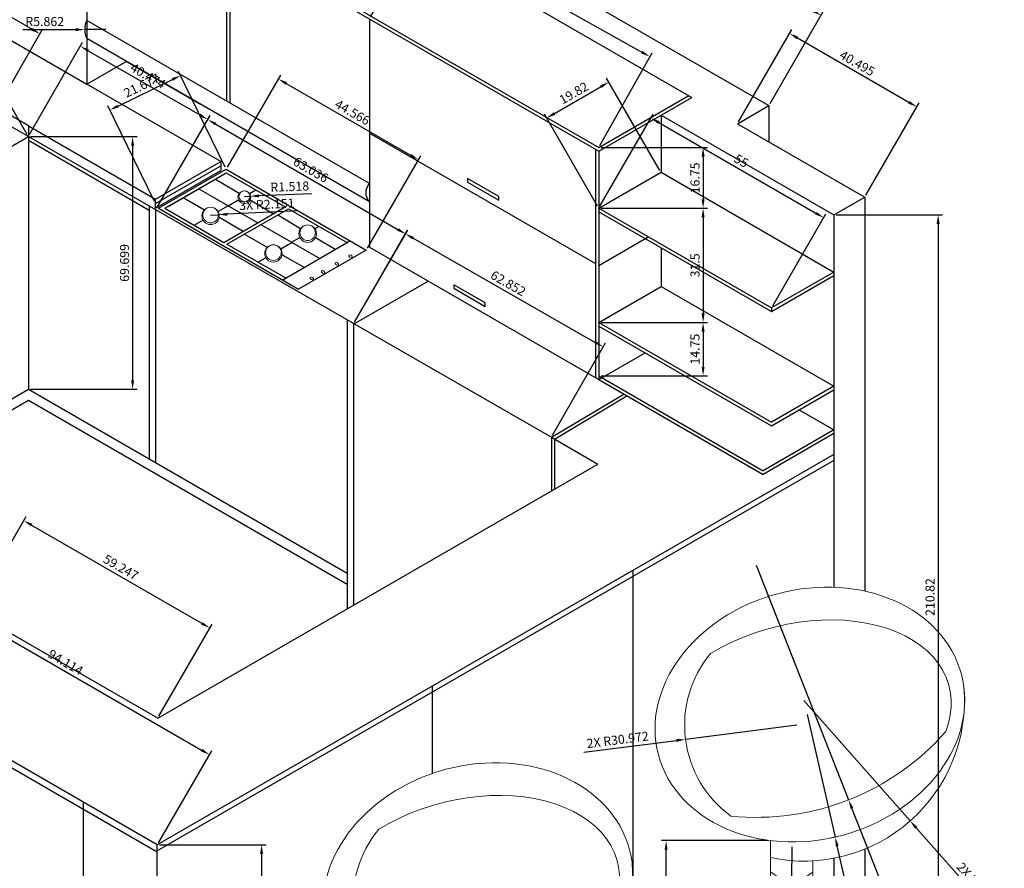
# Model space of a CAD drawing. Units: centimetres. Extents: x 239489 to 240034, y 95136 to 95693.
# Tile 3 of 4: x 239762 to 240034, y 95322 to 95556. Entities that reach past the tile are written whole.
import ezdxf

# ---------------------------------------------------------------- set-up
doc = ezdxf.new("R2010")
doc.units = ezdxf.units.CM
for name, color, linetype, lineweight in [('A-ANNO-DIMS', 2, 'Continuous', 18), ('A-EQPM', 8, 'Continuous', 18), ('A-FLOR-CASE', 7, 'Continuous', 25), ('A-FURN', 8, 'Continuous', 18)]:
    doc.layers.add(name, color=color, linetype=linetype, lineweight=lineweight)
doc.styles.get("Standard").update_dxf_attribs({"font": 'arial.ttf'})
doc.dimstyles.new('ISO-25', dxfattribs={"dimtxt": 2.5, "dimasz": 2.5, "dimexe": 1.25, "dimexo": 0.625, "dimtad": 1, "dimdec": 1, "dimdsep": 46, "dimtxsty": 'Standard', "dimcen": 2.5, "dimadec": 0, "dimazin": 0, "dimtfac": 1, "dimtdec": 1, "dimtmove": 0, "dimatfit": 3, "dimfxl": 1, "dimarcsym": 0})

# ---------------------------------------------------------------- blocks, each defined once
blk = doc.blocks.new('chair')
for p, q in [((240038.62, 95198.57), (240038.62, 95083.6)), ((240050.31, 95192.98), (240050.31, 95083.6))]:
    blk.add_line(p, q)
for centre, radius, start, end in [((240045.95, 95230.38), 30.97, 140.3765, 234.0123), ((240047.85, 95237.18), 44.27, 257.9755, 4.8871), ((240034.71, 95274.51), 69.54, 264.2585, 318.7167), ((240048.77, 95233.37), 34.72, 279.5939, 286.053), ((240044.52, 95196.85), 9.07, 229.4992, 309.6922), ((240044.46, 95080.37), 6.67, 151.0567, 28.8701), ((240044.47, 95082.04), 6.05, 165.0328, 14.894), ((240044.47, 95086.14), 6.37, 203.4476, 336.4791)]:
    blk.add_arc(centre, radius, start, end)
blk.add_ellipse((240049.51, 95233.34), major_axis=(41.76, 11.11), ratio=0.798178)
for centre, major_axis, ratio, start_param, end_param in [((240046.12, 95230.16), (41.76, 11.11), 0.649156, 5.842129, 8.285652), ((240044.64, 95075.07), (-24.53, 0), 0.903861, 4.9602, 10.762393)]:
    blk.add_ellipse(centre, major_axis=major_axis, ratio=ratio, start_param=start_param, end_param=end_param)
for points, knots in [([(240050.31, 95149.47), (240053.45, 95154.4), (240062.71, 95168.9), (240023.27, 95171.77), (240016.58, 95146.62), (240022.37, 95124.99), (240049.4, 95122.25), (240052.18, 95137.64), (240053.6, 95145.49)], [0, 0, 0, 0, 14.382035, 42.295085, 64.991841, 82.938136, 102.944135, 123.773993, 123.773993, 123.773993, 123.773993]), ([(240050.31, 95151.33), (240050.86, 95152.21), (240051.4, 95153.07), (240052.67, 95155.21), (240053.34, 95156.46), (240054.37, 95158.8), (240054.7, 95159.88), (240054.88, 95161.29), (240054.88, 95161.73), (240054.77, 95162.52), (240054.66, 95162.88), (240054.32, 95163.58), (240054.09, 95163.91), (240053.51, 95164.56), (240053.15, 95164.87), (240051.85, 95165.79), (240050.7, 95166.33), (240048.02, 95167.17), (240046.5, 95167.47), (240043.26, 95167.81), (240041.54, 95167.85), (240037.24, 95167.61), (240034.64, 95167.17), (240031.24, 95166.1), (240030.23, 95165.71), (240027.8, 95164.52), (240026.51, 95163.63), (240024.3, 95161.56), (240023.38, 95160.4), (240021.86, 95157.85), (240021.25, 95156.46), (240019.83, 95151.95), (240019.48, 95148.58), (240019.62, 95142.56), (240019.95, 95139.94), (240021.18, 95135.59), (240021.97, 95133.78), (240023.74, 95131.18), (240024.56, 95130.25), (240026.17, 95128.89), (240026.88, 95128.4), (240028.41, 95127.53), (240029.24, 95127.14), (240032.19, 95126.03), (240034.5, 95125.58), (240038.99, 95125.46), (240041.16, 95125.78), (240043.66, 95126.75), (240044.27, 95127.05), (240045.4, 95127.76), (240045.91, 95128.16), (240047.34, 95129.53), (240048.14, 95130.64), (240049.5, 95133.2), (240050.06, 95134.65), (240050.79, 95137.03), (240051.02, 95137.89), (240051.24, 95138.77)], [1.291453, 1.291453, 1.291453, 1.291453, 3.859328, 3.859328, 7.768299, 7.768299, 11.677271, 11.677271, 13.651412, 13.651412, 15.625553, 15.625553, 17.599694, 17.599694, 19.573836, 19.573836, 23.79302, 23.79302, 28.012204, 28.012204, 32.231389, 32.231389, 38.538282, 38.538282, 41.377864, 41.377864, 45.999792, 45.999792, 50.62172, 50.62172, 55.243647, 55.243647, 64.836636, 64.836636, 72.329787, 72.329787, 78.440683, 78.440683, 82.448991, 82.448991, 85.126657, 85.126657, 87.804323, 87.804323, 94.31242, 94.31242, 100.820517, 100.820517, 103.180094, 103.180094, 105.53967, 105.53967, 110.270519, 110.270519, 115.001369, 115.001369, 117.513572, 117.513572, 117.513572, 117.513572]), ([(240038.62, 95150.05), (240037.1, 95148.99), (240030.34, 95144.28), (240045.99, 95138.79), (240055.45, 95146.41), (240051.11, 95148.83), (240050.31, 95149.47)], [0, 0, 0, 0, 4.688566, 20.875909, 24.405284, 27.513147, 27.513147, 27.513147, 27.513147]), ([(240038.62, 95145.45), (240038.41, 95145.3), (240038.2, 95145.16), (240037.99, 95145.01), (240036.47, 95143.95), (240029.7, 95139.25), (240045.36, 95133.75), (240054.55, 95141.16), (240051.25, 95143.33), (240050.31, 95143.98)], [-0.650979, -0.650979, -0.650979, -0.650979, 0, 0, 0, 4.688566, 20.875909, 24.405284, 26.869866, 26.869866, 26.869866, 26.869866])]:
    blk.add_open_spline(points, degree=3, knots=knots)
blk = doc.blocks.new('HANDLE-DOOR')
for p, q in [((0.87, 10.5), (0, 10)), ((0, 10), (0, 0)), ((0.87, 0.5), (0.87, 10.5)), ((0, 0), (0.87, 0.5))]:
    blk.add_line(p, q)
blk = doc.blocks.new('*D5')
at = {"layer": 'A-ANNO-DIMS', "color": 0, "lineweight": -2, "transparency": 16777216}
for p, q in [((239735.57, 95667.89), (239750.25, 95693.33)), ((239751.79, 95691), (239980.86, 95558.75)), ((239968.97, 95533.14), (239983.65, 95558.58))]:
    blk.add_line(p, q, dxfattribs=at)
at = {"layer": 'A-ANNO-DIMS', "color": 0, "transparency": 16777216}
for points in [[(239752, 95691.36), (239751.59, 95690.64), (239749.63, 95692.25)], [(239981.07, 95559.11), (239980.65, 95558.39), (239983.03, 95557.5)]]:
    blk.add_solid(points, dxfattribs=at)
at = {"layer": 'Defpoints', "color": 0, "transparency": 16777216}
for p in [(239735.25, 95667.35), (239983.03, 95557.5), (239968.65, 95532.6)]:
    blk.add_point(p, dxfattribs=at)
at = {"layer": 'A-ANNO-DIMS', "color": 0, "transparency": 16777216, "insert": (239867.28, 95626.52), "char_height": 2.5, "attachment_point": 5, "rotation": 330}
blk.add_mtext('269.505', dxfattribs=at)
blk = doc.blocks.new('*D6')
at = {"layer": 'A-ANNO-DIMS', "color": 0, "lineweight": -2, "transparency": 16777216}
for p, q in [((239960.31, 95528.14), (239974.99, 95553.58)), ((239976.53, 95551.25), (240007.27, 95533.5)), ((239995.37, 95507.89), (240010.06, 95533.33))]:
    blk.add_line(p, q, dxfattribs=at)
at = {"layer": 'A-ANNO-DIMS', "color": 0, "transparency": 16777216}
for points in [[(239976.74, 95551.61), (239976.32, 95550.89), (239974.37, 95552.5)], [(240007.48, 95533.86), (240007.06, 95533.14), (240009.44, 95532.25)]]:
    blk.add_solid(points, dxfattribs=at)
at = {"layer": 'Defpoints', "color": 0, "transparency": 16777216}
for p in [(240009.44, 95532.25), (239959.99, 95527.6), (239995.06, 95507.35)]:
    blk.add_point(p, dxfattribs=at)
at = {"layer": 'A-ANNO-DIMS', "color": 0, "transparency": 16777216, "insert": (239992.85, 95544.02), "char_height": 2.5, "attachment_point": 5, "rotation": 330}
blk.add_mtext('40.495', dxfattribs=at)
blk = doc.blocks.new('*D9')
at = {"layer": 'A-ANNO-DIMS', "color": 0, "lineweight": -2, "transparency": 16777216}
for p, q in [((239987.18, 95502.44), (240016.56, 95502.44)), ((240015.31, 95499.94), (240015.31, 95294.12)), ((239987.18, 95291.62), (240016.56, 95291.62))]:
    blk.add_line(p, q, dxfattribs=at)
at = {"layer": 'A-ANNO-DIMS', "color": 0, "transparency": 16777216}
for points in [[(240014.89, 95499.94), (240015.73, 95499.94), (240015.31, 95502.44)], [(240014.89, 95294.12), (240015.73, 95294.12), (240015.31, 95291.62)]]:
    blk.add_solid(points, dxfattribs=at)
at = {"layer": 'Defpoints', "color": 0, "transparency": 16777216}
for p in [(239986.56, 95502.44), (239986.56, 95291.62), (240015.31, 95291.62)]:
    blk.add_point(p, dxfattribs=at)
at = {"layer": 'A-ANNO-DIMS', "color": 0, "transparency": 16777216, "insert": (240013.41, 95397.03), "char_height": 2.5, "attachment_point": 5, "rotation": 90}
blk.add_mtext('210.82', dxfattribs=at)
blk = doc.blocks.new('*D24')
at = {"layer": 'A-ANNO-DIMS', "color": 0, "lineweight": -2, "transparency": 16777216}
for p, q in [((239858.85, 95557.08), (239873.23, 95582.69)), ((239874.8, 95580.37), (239933.66, 95547.32)), ((239922.07, 95521.58), (239936.45, 95547.19))]:
    blk.add_line(p, q, dxfattribs=at)
at = {"layer": 'A-ANNO-DIMS', "color": 0, "transparency": 16777216}
for points in [[(239875, 95580.74), (239874.6, 95580.01), (239872.62, 95581.6)], [(239933.86, 95547.69), (239933.46, 95546.96), (239935.84, 95546.1)]]:
    blk.add_solid(points, dxfattribs=at)
at = {"layer": 'Defpoints', "color": 0, "transparency": 16777216}
for p in [(239858.54, 95556.53), (239935.84, 95546.1), (239921.76, 95521.03)]:
    blk.add_point(p, dxfattribs=at)
at = {"layer": 'A-ANNO-DIMS', "color": 0, "transparency": 16777216, "insert": (239905.16, 95565.51), "char_height": 2.5, "attachment_point": 5, "rotation": 330.6844}
blk.add_mtext('72.505', dxfattribs=at)
blk = doc.blocks.new('*D25')
at = {"layer": 'A-ANNO-DIMS', "color": 0, "lineweight": -2, "transparency": 16777216}
for p, q in [((239922.39, 95521.03), (239951.76, 95521.03)), ((239950.51, 95518.53), (239950.51, 95506.78)), ((239922.39, 95504.28), (239951.76, 95504.28))]:
    blk.add_line(p, q, dxfattribs=at)
at = {"layer": 'A-ANNO-DIMS', "color": 0, "transparency": 16777216}
for points in [[(239950.1, 95518.53), (239950.93, 95518.53), (239950.51, 95521.03)], [(239950.1, 95506.78), (239950.93, 95506.78), (239950.51, 95504.28)]]:
    blk.add_solid(points, dxfattribs=at)
at = {"layer": 'Defpoints', "color": 0, "transparency": 16777216}
for p in [(239921.76, 95521.03), (239921.76, 95504.28), (239950.51, 95504.28)]:
    blk.add_point(p, dxfattribs=at)
at = {"layer": 'A-ANNO-DIMS', "color": 0, "transparency": 16777216, "insert": (239948.61, 95512.66), "char_height": 2.5, "attachment_point": 5, "rotation": 90}
blk.add_mtext('16.75', dxfattribs=at)
blk = doc.blocks.new('*D26')
at = {"layer": 'A-ANNO-DIMS', "color": 0, "lineweight": -2, "transparency": 16777216}
for p, q in [((239922.39, 95504.28), (239951.76, 95504.28)), ((239950.51, 95501.78), (239950.51, 95475.28)), ((239922.39, 95472.78), (239951.76, 95472.78))]:
    blk.add_line(p, q, dxfattribs=at)
at = {"layer": 'A-ANNO-DIMS', "color": 0, "transparency": 16777216}
for points in [[(239950.1, 95501.78), (239950.93, 95501.78), (239950.51, 95504.28)], [(239950.1, 95475.28), (239950.93, 95475.28), (239950.51, 95472.78)]]:
    blk.add_solid(points, dxfattribs=at)
at = {"layer": 'Defpoints', "color": 0, "transparency": 16777216}
for p in [(239921.76, 95504.28), (239921.76, 95472.78), (239950.51, 95472.78)]:
    blk.add_point(p, dxfattribs=at)
at = {"layer": 'A-ANNO-DIMS', "color": 0, "transparency": 16777216, "insert": (239948.61, 95488.53), "char_height": 2.5, "attachment_point": 5, "rotation": 90}
blk.add_mtext('31.5', dxfattribs=at)
blk = doc.blocks.new('*D27')
at = {"layer": 'A-ANNO-DIMS', "color": 0, "lineweight": -2, "transparency": 16777216}
for p, q in [((239922.39, 95472.78), (239951.76, 95472.78)), ((239950.51, 95470.28), (239950.51, 95460.53)), ((239922.39, 95458.03), (239951.76, 95458.03))]:
    blk.add_line(p, q, dxfattribs=at)
at = {"layer": 'A-ANNO-DIMS', "color": 0, "transparency": 16777216}
for points in [[(239950.1, 95470.28), (239950.93, 95470.28), (239950.51, 95472.78)], [(239950.1, 95460.53), (239950.93, 95460.53), (239950.51, 95458.03)]]:
    blk.add_solid(points, dxfattribs=at)
at = {"layer": 'Defpoints', "color": 0, "transparency": 16777216}
for p in [(239921.76, 95472.78), (239921.76, 95458.03), (239950.51, 95458.03)]:
    blk.add_point(p, dxfattribs=at)
at = {"layer": 'A-ANNO-DIMS', "color": 0, "transparency": 16777216, "insert": (239948.61, 95465.41), "char_height": 2.5, "attachment_point": 5, "rotation": 90}
blk.add_mtext('14.75', dxfattribs=at)
blk = doc.blocks.new('*D28')
at = {"layer": 'A-ANNO-DIMS', "color": 0, "lineweight": -2, "transparency": 16777216}
for p, q in [((239922.08, 95504.82), (239936.76, 95530.26)), ((239938.3, 95527.93), (239981.6, 95502.93)), ((239969.71, 95477.32), (239984.39, 95502.76))]:
    blk.add_line(p, q, dxfattribs=at)
at = {"layer": 'A-ANNO-DIMS', "color": 0, "transparency": 16777216}
for points in [[(239938.51, 95528.29), (239938.09, 95527.57), (239936.14, 95529.18)], [(239981.81, 95503.29), (239981.4, 95502.57), (239983.77, 95501.68)]]:
    blk.add_solid(points, dxfattribs=at)
at = {"layer": 'Defpoints', "color": 0, "transparency": 16777216}
for p in [(239921.76, 95504.28), (239983.77, 95501.68), (239969.39, 95476.78)]:
    blk.add_point(p, dxfattribs=at)
at = {"layer": 'A-ANNO-DIMS', "color": 0, "transparency": 16777216, "insert": (239960.9, 95517.07), "char_height": 2.5, "attachment_point": 5, "rotation": 330}
blk.add_mtext('55', dxfattribs=at)
blk = doc.blocks.new('*D29')
at = {"layer": 'A-ANNO-DIMS', "color": 0, "lineweight": -2, "transparency": 16777216}
for p, q in [((239938.61, 95514.73), (239923.93, 95540.17)), ((239909.55, 95530.43), (239922.39, 95537.84)), ((239921.45, 95504.82), (239906.76, 95530.26))]:
    blk.add_line(p, q, dxfattribs=at)
at = {"layer": 'A-ANNO-DIMS', "color": 0, "transparency": 16777216}
for points in [[(239922.18, 95538.2), (239922.6, 95537.48), (239924.55, 95539.09)], [(239909.34, 95530.79), (239909.76, 95530.07), (239907.39, 95529.18)]]:
    blk.add_solid(points, dxfattribs=at)
at = {"layer": 'Defpoints', "color": 0, "transparency": 16777216}
for p in [(239924.55, 95539.09), (239938.93, 95514.19), (239921.76, 95504.28)]:
    blk.add_point(p, dxfattribs=at)
at = {"layer": 'A-ANNO-DIMS', "color": 0, "transparency": 16777216, "insert": (239915.02, 95535.78), "char_height": 2.5, "attachment_point": 5, "rotation": 30}
blk.add_mtext('19.82', dxfattribs=at)
blk = doc.blocks.new('*D32')
at = {"layer": 'A-ANNO-DIMS', "color": 0, "lineweight": -2, "transparency": 16777216}
for p, q in [((239764.18, 95524.59), (239749.49, 95550.03)), ((239697.39, 95518.51), (239747.95, 95547.7)), ((239709.29, 95492.9), (239694.6, 95518.34))]:
    blk.add_line(p, q, dxfattribs=at)
at = {"layer": 'A-ANNO-DIMS', "color": 0, "transparency": 16777216}
for points in [[(239747.75, 95548.06), (239748.16, 95547.34), (239750.12, 95548.95)], [(239697.19, 95518.87), (239697.6, 95518.15), (239695.23, 95517.26)]]:
    blk.add_solid(points, dxfattribs=at)
at = {"layer": 'Defpoints', "color": 0, "transparency": 16777216}
for p in [(239750.12, 95548.95), (239764.49, 95524.05), (239709.6, 95492.36)]:
    blk.add_point(p, dxfattribs=at)
at = {"layer": 'A-ANNO-DIMS', "color": 0, "transparency": 16777216, "insert": (239721.72, 95534.75), "char_height": 2.5, "attachment_point": 5, "rotation": 30}
blk.add_mtext('63.381', dxfattribs=at)
blk = doc.blocks.new('*D33')
at = {"layer": 'A-ANNO-DIMS', "color": 0, "lineweight": -2, "transparency": 16777216}
for p, q in [((239764.81, 95524.59), (239779.45, 95550.06)), ((239781, 95547.73), (239811.75, 95530.04)), ((239799.89, 95504.41), (239814.54, 95529.87))]:
    blk.add_line(p, q, dxfattribs=at)
at = {"layer": 'A-ANNO-DIMS', "color": 0, "transparency": 16777216}
for points in [[(239781.21, 95548.09), (239780.79, 95547.36), (239778.83, 95548.97)], [(239811.95, 95530.4), (239811.54, 95529.67), (239813.91, 95528.79)]]:
    blk.add_solid(points, dxfattribs=at)
at = {"layer": 'Defpoints', "color": 0, "transparency": 16777216}
for p in [(239813.91, 95528.79), (239764.49, 95524.05), (239799.58, 95503.87)]:
    blk.add_point(p, dxfattribs=at)
at = {"layer": 'A-ANNO-DIMS', "color": 0, "transparency": 16777216, "insert": (239797.32, 95540.53), "char_height": 2.5, "attachment_point": 5, "rotation": 330.0888}
blk.add_mtext('40.474', dxfattribs=at)
blk = doc.blocks.new('*D34')
at = {"layer": 'A-ANNO-DIMS', "color": 0, "lineweight": -2, "transparency": 16777216}
for p, q in [((239799.89, 95504.41), (239814.6, 95529.83)), ((239816.14, 95527.5), (239866.37, 95498.43)), ((239854.45, 95472.84), (239869.16, 95498.26))]:
    blk.add_line(p, q, dxfattribs=at)
at = {"layer": 'A-ANNO-DIMS', "color": 0, "transparency": 16777216}
for points in [[(239816.35, 95527.86), (239815.93, 95527.14), (239813.98, 95528.75)], [(239866.58, 95498.79), (239866.16, 95498.07), (239868.54, 95497.18)]]:
    blk.add_solid(points, dxfattribs=at)
at = {"layer": 'Defpoints', "color": 0, "transparency": 16777216}
for p in [(239799.58, 95503.87), (239868.54, 95497.18), (239854.14, 95472.3)]:
    blk.add_point(p, dxfattribs=at)
at = {"layer": 'A-ANNO-DIMS', "color": 0, "transparency": 16777216, "insert": (239842.21, 95514.61), "char_height": 2.5, "attachment_point": 5, "rotation": 329.943}
blk.add_mtext('63.036', dxfattribs=at)
blk = doc.blocks.new('*D35')
at = {"layer": 'A-ANNO-DIMS', "color": 0, "lineweight": -2, "transparency": 16777216}
for p, q in [((239854.45, 95472.84), (239869.03, 95498.34)), ((239870.58, 95496.01), (239920.8, 95467.29)), ((239909.01, 95441.64), (239923.59, 95467.14))]:
    blk.add_line(p, q, dxfattribs=at)
at = {"layer": 'A-ANNO-DIMS', "color": 0, "transparency": 16777216}
for points in [[(239870.79, 95496.37), (239870.37, 95495.65), (239868.41, 95497.25)], [(239921.01, 95467.65), (239920.59, 95466.93), (239922.97, 95466.05)]]:
    blk.add_solid(points, dxfattribs=at)
at = {"layer": 'Defpoints', "color": 0, "transparency": 16777216}
for p in [(239854.14, 95472.3), (239922.97, 95466.05), (239908.7, 95441.09)]:
    blk.add_point(p, dxfattribs=at)
at = {"layer": 'A-ANNO-DIMS', "color": 0, "transparency": 16777216, "insert": (239896.63, 95483.3), "char_height": 2.5, "attachment_point": 5, "rotation": 330.235}
blk.add_mtext('62.852', dxfattribs=at)
blk = doc.blocks.new('*D36')
at = {"layer": 'A-ANNO-DIMS', "color": 0, "lineweight": -2, "transparency": 16777216}
for p, q in [((239765.12, 95524.05), (239794.49, 95524.05)), ((239793.24, 95521.55), (239793.24, 95456.85)), ((239765.12, 95454.35), (239794.49, 95454.35))]:
    blk.add_line(p, q, dxfattribs=at)
at = {"layer": 'A-ANNO-DIMS', "color": 0, "transparency": 16777216}
for points in [[(239792.83, 95521.55), (239793.66, 95521.55), (239793.24, 95524.05)], [(239792.83, 95456.85), (239793.66, 95456.85), (239793.24, 95454.35)]]:
    blk.add_solid(points, dxfattribs=at)
at = {"layer": 'Defpoints', "color": 0, "transparency": 16777216}
for p in [(239764.49, 95524.05), (239764.49, 95454.35), (239793.24, 95454.35)]:
    blk.add_point(p, dxfattribs=at)
at = {"layer": 'A-ANNO-DIMS', "color": 0, "transparency": 16777216, "insert": (239791.34, 95489.2), "char_height": 2.5, "attachment_point": 5, "rotation": 90}
blk.add_mtext('69.699', dxfattribs=at)
blk = doc.blocks.new('*D39')
at = {"layer": 'A-ANNO-DIMS', "color": 0, "lineweight": -2, "transparency": 16777216}
for p, q in [((239717.29, 95549.03), (239731.97, 95574.47)), ((239733.51, 95572.13), (239765.51, 95553.66)), ((239753.61, 95528.06), (239768.3, 95553.5))]:
    blk.add_line(p, q, dxfattribs=at)
at = {"layer": 'A-ANNO-DIMS', "color": 0, "transparency": 16777216}
for points in [[(239733.72, 95572.5), (239733.31, 95571.77), (239731.35, 95573.38)], [(239765.72, 95554.02), (239765.3, 95553.3), (239767.67, 95552.41)]]:
    blk.add_solid(points, dxfattribs=at)
at = {"layer": 'Defpoints', "color": 0, "transparency": 16777216}
for p in [(239767.67, 95552.41), (239716.97, 95548.49), (239753.3, 95527.52)]:
    blk.add_point(p, dxfattribs=at)
at = {"layer": 'A-ANNO-DIMS', "color": 0, "transparency": 16777216, "insert": (239750.46, 95564.55), "char_height": 2.5, "attachment_point": 5, "rotation": 330}
blk.add_mtext('41.943', dxfattribs=at)
blk = doc.blocks.new('*D40')
at = {"layer": 'A-ANNO-DIMS', "color": 0, "lineweight": -2, "transparency": 16777216}
for p, q in [((239818.79, 95515.61), (239805.92, 95542.01)), ((239789.22, 95532.48), (239804.22, 95539.79)), ((239799.3, 95506.11), (239786.43, 95532.51))]:
    blk.add_line(p, q, dxfattribs=at)
at = {"layer": 'A-ANNO-DIMS', "color": 0, "transparency": 16777216}
for points in [[(239804.03, 95540.17), (239804.4, 95539.42), (239806.46, 95540.89)], [(239789.04, 95532.86), (239789.41, 95532.11), (239786.98, 95531.39)]]:
    blk.add_solid(points, dxfattribs=at)
at = {"layer": 'Defpoints', "color": 0, "transparency": 16777216}
for p in [(239806.46, 95540.89), (239819.06, 95515.05), (239799.58, 95505.55)]:
    blk.add_point(p, dxfattribs=at)
at = {"layer": 'A-ANNO-DIMS', "color": 0, "transparency": 16777216, "insert": (239795.89, 95537.85), "char_height": 2.5, "attachment_point": 5, "rotation": 25.9908}
blk.add_mtext('21.677', dxfattribs=at)
blk = doc.blocks.new('*D41')
at = {"layer": 'A-ANNO-DIMS', "color": 0, "lineweight": -2, "transparency": 16777216}
for p, q in [((239819.37, 95515.59), (239834.06, 95541.03)), ((239835.6, 95538.69), (239869.87, 95518.91)), ((239857.97, 95493.3), (239872.66, 95518.74))]:
    blk.add_line(p, q, dxfattribs=at)
at = {"layer": 'A-ANNO-DIMS', "color": 0, "transparency": 16777216}
for points in [[(239835.81, 95539.06), (239835.39, 95538.33), (239833.44, 95539.94)], [(239870.08, 95519.27), (239869.66, 95518.55), (239872.03, 95517.66)]]:
    blk.add_solid(points, dxfattribs=at)
at = {"layer": 'Defpoints', "color": 0, "transparency": 16777216}
for p in [(239872.03, 95517.66), (239819.06, 95515.05), (239857.66, 95492.76)]:
    blk.add_point(p, dxfattribs=at)
at = {"layer": 'A-ANNO-DIMS', "color": 0, "transparency": 16777216, "insert": (239853.69, 95530.45), "char_height": 2.5, "attachment_point": 5, "rotation": 330}
blk.add_mtext('44.566', dxfattribs=at)
blk = doc.blocks.new('*D42')
at = {"layer": 'A-ANNO-DIMS', "color": 0, "lineweight": -2, "transparency": 16777216}
for p, q in [((239800.67, 95328.67), (239830.05, 95328.67)), ((239828.8, 95326.17), (239828.8, 95186.44)), ((239800.67, 95183.94), (239830.05, 95183.94))]:
    blk.add_line(p, q, dxfattribs=at)
at = {"layer": 'A-ANNO-DIMS', "color": 0, "transparency": 16777216}
for points in [[(239828.38, 95326.17), (239829.22, 95326.17), (239828.8, 95328.67)], [(239828.38, 95186.44), (239829.22, 95186.44), (239828.8, 95183.94)]]:
    blk.add_solid(points, dxfattribs=at)
at = {"layer": 'Defpoints', "color": 0, "transparency": 16777216}
for p in [(239800.05, 95328.67), (239800.05, 95183.94), (239828.8, 95183.94)]:
    blk.add_point(p, dxfattribs=at)
at = {"layer": 'A-ANNO-DIMS', "color": 0, "transparency": 16777216, "insert": (239826.9, 95256.31), "char_height": 2.5, "attachment_point": 5, "rotation": 90}
blk.add_mtext('144.73', dxfattribs=at)
blk = doc.blocks.new('*D44')
at = {"layer": 'A-ANNO-DIMS', "color": 0, "lineweight": -2, "transparency": 16777216}
for p, q in [((239718.86, 95376.27), (239733.54, 95401.71)), ((239735.08, 95399.38), (239812.26, 95354.82)), ((239800.36, 95329.21), (239815.05, 95354.65))]:
    blk.add_line(p, q, dxfattribs=at)
at = {"layer": 'A-ANNO-DIMS', "color": 0, "transparency": 16777216}
for points in [[(239735.29, 95399.74), (239734.88, 95399.02), (239732.92, 95400.63)], [(239812.47, 95355.18), (239812.05, 95354.46), (239814.42, 95353.57)]]:
    blk.add_solid(points, dxfattribs=at)
at = {"layer": 'Defpoints', "color": 0, "transparency": 16777216}
for p in [(239718.54, 95375.73), (239814.42, 95353.57), (239800.05, 95328.67)]:
    blk.add_point(p, dxfattribs=at)
at = {"layer": 'A-ANNO-DIMS', "color": 0, "transparency": 16777216, "insert": (239774.62, 95378.75), "char_height": 2.5, "attachment_point": 5, "rotation": 330}
blk.add_mtext('94.114', dxfattribs=at)
blk = doc.blocks.new('*D46')
at = {"layer": 'A-ANNO-DIMS', "color": 0, "lineweight": -2, "transparency": 16777216}
for p, q in [((239749.17, 95393.77), (239763.86, 95419.21)), ((239765.4, 95416.88), (239812.38, 95389.75)), ((239800.48, 95364.15), (239815.17, 95389.59))]:
    blk.add_line(p, q, dxfattribs=at)
at = {"layer": 'A-ANNO-DIMS', "color": 0, "transparency": 16777216}
for points in [[(239765.6, 95417.24), (239765.19, 95416.52), (239763.23, 95418.13)], [(239812.58, 95390.11), (239812.17, 95389.39), (239814.54, 95388.5)]]:
    blk.add_solid(points, dxfattribs=at)
at = {"layer": 'Defpoints', "color": 0, "transparency": 16777216}
for p in [(239748.86, 95393.23), (239814.54, 95388.5), (239800.17, 95363.61)]:
    blk.add_point(p, dxfattribs=at)
at = {"layer": 'A-ANNO-DIMS', "color": 0, "transparency": 16777216, "insert": (239789.84, 95404.96), "char_height": 2.5, "attachment_point": 5, "rotation": 330}
blk.add_mtext('59.247', dxfattribs=at)
blk = doc.blocks.new('*D47')
at = {"layer": 'A-ANNO-DIMS', "color": 0, "lineweight": -2, "transparency": 16777216}
for p, q in [((239968.45, 95329.85), (239939.07, 95329.85)), ((239940.32, 95217.39), (239940.32, 95327.35)), ((239968.45, 95214.89), (239939.07, 95214.89))]:
    blk.add_line(p, q, dxfattribs=at)
at = {"layer": 'A-ANNO-DIMS', "color": 0, "transparency": 16777216}
for points in [[(239939.91, 95327.35), (239940.74, 95327.35), (239940.32, 95329.85)], [(239939.91, 95217.39), (239940.74, 95217.39), (239940.32, 95214.89)]]:
    blk.add_solid(points, dxfattribs=at)
at = {"layer": 'Defpoints', "color": 0, "transparency": 16777216}
for p in [(239940.32, 95329.85), (239969.07, 95329.85), (239969.07, 95214.89)]:
    blk.add_point(p, dxfattribs=at)
at = {"layer": 'A-ANNO-DIMS', "color": 0, "transparency": 16777216, "insert": (239938.42, 95272.37), "char_height": 2.5, "attachment_point": 5, "rotation": 90}
blk.add_mtext('114.968', dxfattribs=at)
blk = doc.blocks.new('*D49')
at = {"layer": 'A-ANNO-DIMS', "color": 0, "lineweight": -2, "transparency": 16777216}
for p, q in [((239814.73, 95502.4), (239816.88, 95502.51)), ((239838.82, 95503.54), (239819.38, 95502.62))]:
    blk.add_line(p, q, dxfattribs=at)
at = {"layer": 'A-ANNO-DIMS', "color": 0, "transparency": 16777216}
blk.add_solid([(239819.36, 95503.04), (239819.4, 95502.21), (239816.88, 95502.51)], dxfattribs=at)
at = {"layer": 'Defpoints', "color": 0, "transparency": 16777216}
for p in [(239814.73, 95502.4), (239816.88, 95502.51)]:
    blk.add_point(p, dxfattribs=at)
at = {"layer": 'A-ANNO-DIMS', "color": 0, "transparency": 16777216, "insert": (239830.26, 95505.04), "char_height": 2.5, "attachment_point": 5, "rotation": 2.7081}
blk.add_mtext('3X R2.151', dxfattribs=at)
blk = doc.blocks.new('*D50')
at = {"layer": 'A-ANNO-DIMS', "color": 0, "lineweight": -2, "transparency": 16777216}
for p, q in [((239824.09, 95507.56), (239825.6, 95507.61)), ((239842.68, 95508.24), (239828.1, 95507.7))]:
    blk.add_line(p, q, dxfattribs=at)
at = {"layer": 'A-ANNO-DIMS', "color": 0, "transparency": 16777216}
blk.add_solid([(239828.09, 95508.12), (239828.12, 95507.29), (239825.6, 95507.61)], dxfattribs=at)
at = {"layer": 'Defpoints', "color": 0, "transparency": 16777216}
for p in [(239824.09, 95507.56), (239825.6, 95507.61)]:
    blk.add_point(p, dxfattribs=at)
at = {"layer": 'A-ANNO-DIMS', "color": 0, "transparency": 16777216, "insert": (239836.57, 95509.92), "char_height": 2.5, "attachment_point": 5, "rotation": 2.1233}
blk.add_mtext('R1.518', dxfattribs=at)
blk = doc.blocks.new('*D51')
at = {"layer": 'A-ANNO-DIMS', "color": 0, "lineweight": -2, "transparency": 16777216}
for p, q in [((239762.99, 95553.56), (239777.54, 95553.56)), ((239785.9, 95553.56), (239780.04, 95553.56))]:
    blk.add_line(p, q, dxfattribs=at)
at = {"layer": 'A-ANNO-DIMS', "color": 0, "transparency": 16777216}
blk.add_solid([(239777.54, 95553.98), (239777.54, 95553.15), (239780.04, 95553.56)], dxfattribs=at)
at = {"layer": 'Defpoints', "color": 0, "transparency": 16777216}
for p in [(239780.04, 95553.56), (239785.9, 95553.56)]:
    blk.add_point(p, dxfattribs=at)
at = {"layer": 'A-ANNO-DIMS', "color": 0, "transparency": 16777216, "insert": (239769.01, 95555.46), "char_height": 2.5, "attachment_point": 5, "rotation": 0.0036}
blk.add_mtext('R5.862', dxfattribs=at)
blk = doc.blocks.new('*D52')
at = {"layer": 'A-ANNO-DIMS', "color": 0, "lineweight": -2, "transparency": 16777216}
for p, q in [((239965.16, 95405.79), (239990.63, 95341.09)), ((240009.47, 95293.22), (239991.54, 95338.76))]:
    blk.add_line(p, q, dxfattribs=at)
at = {"layer": 'A-ANNO-DIMS', "color": 0, "transparency": 16777216}
blk.add_solid([(239991.93, 95338.91), (239991.16, 95338.61), (239990.63, 95341.09)], dxfattribs=at)
at = {"layer": 'Defpoints', "color": 0, "transparency": 16777216}
for p in [(239965.16, 95405.79), (239990.63, 95341.09)]:
    blk.add_point(p, dxfattribs=at)
at = {"layer": 'A-ANNO-DIMS', "color": 0, "transparency": 16777216, "insert": (240007.68, 95302.96), "char_height": 2.5, "attachment_point": 5, "rotation": 291.4873}
blk.add_mtext('2X R69.537', dxfattribs=at)
blk = doc.blocks.new('*D53')
at = {"layer": 'A-ANNO-DIMS', "color": 0, "lineweight": -2, "transparency": 16777216}
for p, q in [((239978.3, 95368.47), (240007.59, 95335.27)), ((240031.61, 95308.06), (240009.25, 95333.4))]:
    blk.add_line(p, q, dxfattribs=at)
at = {"layer": 'A-ANNO-DIMS', "color": 0, "transparency": 16777216}
blk.add_solid([(240009.56, 95333.67), (240008.94, 95333.12), (240007.59, 95335.27)], dxfattribs=at)
at = {"layer": 'Defpoints', "color": 0, "transparency": 16777216}
for p in [(239978.3, 95368.47), (240007.59, 95335.27)]:
    blk.add_point(p, dxfattribs=at)
at = {"layer": 'A-ANNO-DIMS', "color": 0, "transparency": 16777216, "insert": (240026.6, 95316.61), "char_height": 2.5, "attachment_point": 5, "rotation": 311.4309}
blk.add_mtext('2X R44.275', dxfattribs=at)
blk = doc.blocks.new('*D54')
at = {"layer": 'A-ANNO-DIMS', "color": 0, "lineweight": -2, "transparency": 16777216}
for p, q in [((239979.22, 95364.65), (239986.93, 95330.8)), ((239993.71, 95301.02), (239987.48, 95328.36))]:
    blk.add_line(p, q, dxfattribs=at)
at = {"layer": 'A-ANNO-DIMS', "color": 0, "transparency": 16777216}
blk.add_solid([(239987.89, 95328.45), (239987.08, 95328.27), (239986.93, 95330.8)], dxfattribs=at)
at = {"layer": 'Defpoints', "color": 0, "transparency": 16777216}
for p in [(239979.22, 95364.65), (239986.93, 95330.8)]:
    blk.add_point(p, dxfattribs=at)
at = {"layer": 'A-ANNO-DIMS', "color": 0, "transparency": 16777216, "insert": (239993.41, 95310.91), "char_height": 2.5, "attachment_point": 5, "rotation": 282.8235}
blk.add_mtext('2X R34.722', dxfattribs=at)
blk = doc.blocks.new('*D55')
at = {"layer": 'A-ANNO-DIMS', "color": 0, "lineweight": -2, "transparency": 16777216}
for p, q in [((239976.4, 95361.66), (239945.67, 95357.78)), ((239917.61, 95354.24), (239943.19, 95357.47))]:
    blk.add_line(p, q, dxfattribs=at)
at = {"layer": 'A-ANNO-DIMS', "color": 0, "transparency": 16777216}
blk.add_solid([(239943.14, 95357.88), (239943.25, 95357.06), (239945.67, 95357.78)], dxfattribs=at)
at = {"layer": 'Defpoints', "color": 0, "transparency": 16777216}
for p in [(239976.4, 95361.66), (239945.67, 95357.78)]:
    blk.add_point(p, dxfattribs=at)
at = {"layer": 'A-ANNO-DIMS', "color": 0, "transparency": 16777216, "insert": (239927, 95357.34), "char_height": 2.5, "attachment_point": 5, "rotation": 7.1947}
blk.add_mtext('2X R30.972', dxfattribs=at)
blk = doc.blocks.new('*D56')
at = {"layer": 'A-ANNO-DIMS', "color": 0, "lineweight": -2, "transparency": 16777216}
for p, q in [((239974.96, 95328.13), (239974.9, 95319.06)), ((239974.75, 95298.51), (239974.88, 95316.56))]:
    blk.add_line(p, q, dxfattribs=at)
at = {"layer": 'A-ANNO-DIMS', "color": 0, "transparency": 16777216}
blk.add_solid([(239974.46, 95316.57), (239975.3, 95316.56), (239974.9, 95319.06)], dxfattribs=at)
at = {"layer": 'Defpoints', "color": 0, "transparency": 16777216}
for p in [(239974.96, 95328.13), (239974.9, 95319.06)]:
    blk.add_point(p, dxfattribs=at)
at = {"layer": 'A-ANNO-DIMS', "color": 0, "transparency": 16777216, "insert": (239972.91, 95306.3), "char_height": 2.5, "attachment_point": 5, "rotation": 89.593}
blk.add_mtext('2X R9.07', dxfattribs=at)

msp = doc.modelspace()

# ---------------------------------------------------------------- linework, layer by layer
at = {"layer": 'A-ANNO-DIMS'}
for p in [(239921.7628, 95504.2806), (239921.7628, 95488.5306), (239921.7628, 95472.7806)]:
    msp.add_point(p, dxfattribs=at)
at = {"layer": 'A-EQPM'}
for centre, radius in [((239824.0395, 95507.3097), 1.7678), ((239824.0873, 95507.555), 1.5178), ((239814.7335, 95502.1546), 2.4009), ((239814.7335, 95502.4046), 2.1509), ((239841.5023, 95497.2617), 2.4009), ((239841.5023, 95497.5117), 2.1509), ((239832.0552, 95491.8074), 2.4009), ((239832.0552, 95492.0574), 2.1509)]:
    msp.add_circle(centre, radius, dxfattribs=at)
for centre in [(239853.3038, 95491.0662), (239849.5746, 95488.9131), (239845.7472, 95486.7034), (239842.6388, 95484.9087)]:
    msp.add_ellipse(centre, major_axis=(-0.4531, 0.2616), ratio=0.63064412, start_param=-1.57079633, end_param=4.71238898, dxfattribs=at)
at = {"layer": 'A-FLOR-CASE'}
for p, q in [((239735.2548, 95667.3502), (239968.6531, 95532.5976)), ((239735.2548, 95657.3502), (239947.431, 95534.8502)), ((239735.5673, 95628.5306), (239921.7628, 95521.0306)), ((239735.5673, 95627.5306), (239921.7628, 95520.0306)), ((239780.6006, 95601.5306), (239780.6006, 95538.5306)), ((239819.1388, 95579.2806), (239819.1388, 95533.8134)), ((239820.0048, 95578.7806), (239820.0048, 95533.3134)), ((239735.5673, 95564.5306), (239780.6006, 95538.5306)), ((239858.5429, 95556.5306), (239858.5429, 95493.5306)), ((239764.4941, 95527.0512), (239717.5726, 95554.1414)), ((239858.5429, 95511.0634), (239780.6006, 95556.0634)), ((239764.4941, 95524.0512), (239714.9746, 95552.6414)), ((239858.5429, 95506.0634), (239780.6006, 95551.0634)), ((239780.6006, 95538.5306), (239791.4543, 95544.797)), ((239811.9868, 95532.9426), (239791.4543, 95544.797)), ((239817.5715, 95517.1855), (239780.6006, 95538.5306)), ((239921.7628, 95521.0306), (239946.565, 95535.3502)), ((239921.7628, 95520.0306), (239947.431, 95534.8502)), ((239959.9928, 95527.5976), (239968.6531, 95532.5976)), ((239968.6531, 95532.5976), (239968.6531, 95522.5976)), ((239938.927, 95529.9404), (239986.5584, 95502.4404)), ((239938.927, 95529.9404), (239938.927, 95514.1904)), ((239764.4941, 95527.0512), (239799.5768, 95506.7962)), ((239764.4941, 95527.0512), (239764.4941, 95524.0512)), ((239959.9928, 95527.5976), (239995.0624, 95507.3502)), ((239624.4036, 95443.1699), (239764.4941, 95524.0512)), ((239764.4941, 95524.0512), (239908.696, 95441.0939)), ((239764.4941, 95524.0512), (239764.4941, 95454.352)), ((239858.5429, 95525.0306), (239920.8967, 95489.0306)), ((239764.4941, 95523.0512), (239797.8448, 95503.7962)), ((239920.8967, 95520.5306), (239920.8967, 95457.5306)), ((239921.7628, 95520.0306), (239921.7628, 95457.0306)), ((239799.5768, 95506.7962), (239817.5715, 95517.1855)), ((239799.5768, 95505.5463), (239817.5715, 95515.9356)), ((239817.5715, 95517.1855), (239817.5715, 95514.6856)), ((239799.5768, 95504.2964), (239817.5715, 95514.6856)), ((239800.396, 95504.2692), (239819.0619, 95515.0459)), ((239803.0409, 95504.7962), (239819.0619, 95514.0459)), ((239819.0619, 95515.0459), (239857.657, 95492.763)), ((239819.0619, 95514.0459), (239835.3299, 95504.6536)), ((239921.7628, 95504.2806), (239938.927, 95514.1904)), ((239938.927, 95514.1904), (239986.5584, 95486.6904)), ((239802.128, 95504.2692), (239813.7601, 95510.9849)), ((239816.0933, 95512.332), (239822.6561, 95508.4103)), ((239811.4844, 95509.6711), (239827.7524, 95500.2787)), ((239825.4674, 95508.3518), (239827.1959, 95509.3498)), ((239986.5584, 95502.4404), (239995.0624, 95507.3502)), ((239995.0624, 95507.3502), (239995.0624, 95398.6711)), ((239797.8448, 95504.8651), (239797.8448, 95435.097)), ((239799.5768, 95504.2964), (239799.5768, 95506.7962)), ((239813.064, 95503.7607), (239807.1557, 95507.1719)), ((239819.6184, 95504.9749), (239816.8128, 95503.3551)), ((239818.3961, 95494.8768), (239835.3299, 95504.6536)), ((239819.6184, 95504.9749), (239822.423, 95506.5941)), ((239825.6641, 95506.6128), (239832.0814, 95502.7781)), ((239799.5768, 95503.8686), (239799.5768, 95434.097)), ((239800.396, 95504.2692), (239838.9911, 95481.9863)), ((239802.128, 95504.2692), (239818.3961, 95494.8768)), ((239819.2621, 95494.3768), (239836.1959, 95504.1536)), ((239833.2313, 95502.4419), (239839.5597, 95498.6725)), ((239836.1959, 95504.1536), (239852.464, 95494.7612)), ((239921.7628, 95504.2806), (239969.3942, 95476.7806)), ((239921.7628, 95503.2806), (239969.3942, 95475.7806)), ((239986.5584, 95502.4404), (239986.5584, 95399.724)), ((239812.6543, 95500.9542), (239810.262, 95499.573)), ((239817.1087, 95501.8042), (239823.7516, 95497.9689)), ((239828.6185, 95499.7787), (239844.8865, 95490.3864)), ((239843.4648, 95498.6448), (239844.6108, 95499.3064)), ((239830.3857, 95493.4136), (239823.9947, 95497.1092)), ((239819.2621, 95494.3768), (239835.5301, 95484.9845)), ((239837.2199, 95494.8127), (239834.1345, 95493.0079)), ((239853.33, 95495.2612), (239834.6641, 95484.4845)), ((239837.0334, 95494.9316), (239839.3233, 95496.2536)), ((239843.6651, 95496.2193), (239849.2298, 95492.894)), ((239921.7628, 95488.5306), (239935.4027, 95496.4056)), ((239834.4304, 95491.457), (239840.5856, 95487.9033)), ((239857.657, 95492.763), (239838.9911, 95481.9863)), ((239858.5429, 95493.5306), (239966.1991, 95431.3753)), ((239938.927, 95493.3708), (239938.927, 95482.6904)), ((239829.976, 95490.607), (239827.8838, 95489.3991)), ((239986.5584, 95486.6904), (239969.3942, 95476.7806)), ((239969.3942, 95475.7806), (239986.5584, 95485.6904)), ((239854.1364, 95472.2962), (239874.7292, 95484.1855)), ((239921.7628, 95472.7806), (239938.927, 95482.6904)), ((239938.927, 95482.6904), (239986.5584, 95455.1904)), ((239969.3942, 95476.7806), (239969.3942, 95475.7806)), ((239852.4044, 95473.2962), (239852.4044, 95393.7659)), ((239854.1364, 95472.2962), (239854.1364, 95394.7659)), ((239921.7628, 95472.7806), (239969.3942, 95445.2806)), ((239921.7628, 95471.7806), (239969.3942, 95444.2806)), ((239921.7628, 95457.0306), (239934.5366, 95464.4056)), ((239921.7628, 95458.0306), (239967.0651, 95431.8753)), ((239921.7628, 95457.0306), (239967.0651, 95430.8753)), ((239744.7811, 95442.9707), (239764.4941, 95454.352)), ((239764.4941, 95454.352), (239852.4044, 95403.597)), ((239908.696, 95441.0939), (239928.6765, 95453.0389)), ((239986.5584, 95455.1904), (239969.3942, 95445.2806)), ((239969.3942, 95444.2806), (239986.5584, 95454.1904)), ((239624.4036, 95370.4707), (239764.4941, 95451.352)), ((239764.4941, 95451.352), (239852.4044, 95400.597)), ((239909.5469, 95440.6026), (239929.5275, 95452.5476)), ((239976.9796, 95448.6601), (239986.5584, 95443.1297)), ((239986.5584, 95443.1297), (239967.0651, 95431.8753)), ((239908.696, 95441.0939), (239908.696, 95426.2659)), ((239908.696, 95441.0939), (239921.5374, 95433.6799)), ((239909.562, 95440.6116), (239909.562, 95426.7659)), ((239986.5584, 95442.1297), (239967.0651, 95430.8753)), ((239986.5584, 95436.3531), (239800.0497, 95328.6722)), ((239986.5584, 95434.7198), (239800.0497, 95327.0389)), ((239800.1652, 95363.6056), (239921.5374, 95433.6799)), ((239931.1756, 95404.3778), (239931.1756, 95259.6464)), ((239800.1652, 95363.6056), (239748.8555, 95393.2293)), ((239800.0497, 95328.6722), (239718.5446, 95375.7293)), ((239800.0497, 95326.6722), (239718.5446, 95373.7293)), ((239875.7928, 95372.4025), (239875.7928, 95348.3386)), ((239779.6981, 95195.6908), (239779.6981, 95340.4222)), ((239800.0497, 95183.9408), (239800.0497, 95328.6722)), ((239986.5584, 95330.7354), (239986.5584, 95330.716)), ((239995.0624, 95327.4906), (239995.0624, 95296.5314)), ((239986.5584, 95324.9711), (239986.5584, 95291.6216))]:
    msp.add_line(p, q, dxfattribs=at)
for centre, radius, start, end in [((239785.9025, 95553.5634), 5.8617, 154.754596, 205.245404), ((239861.0348, 95508.5634), 3.5298, 134.907237, 225.092763)]:
    msp.add_arc(centre, radius, start, end, dxfattribs=at)

# ---------------------------------------------------------------- block references
for p, rotation in [((239894.2223, 95506.514), 60.00000000004291), ((239890.4432, 95477.1959), 60.00000000045363)]:
    msp.add_blockref('HANDLE-DOOR', p, dxfattribs=dict(at, rotation=rotation))
at = {"layer": 'A-FURN'}
for p in [(-69.552, 131.2835), (-161.0124, 82.8431)]:
    msp.add_blockref('chair', p, dxfattribs=at)

# ---------------------------------------------------------------- dimensions: what is measured, and where the dimension line sits
at = {"layer": 'A-ANNO-DIMS'}
for base, p1, p2, angle, override, picture, middle in [((239983.0281, 95557.4959), (239735.2548, 95667.3502), (239968.6531, 95532.5976), 330, {"dimdec": 3, "dimlfac": 1, "dimrnd": 0, "dimzin": 0, "dimdsep": 46, "dimlunit": 2}, '*D5', (239867.2796, 95626.5188)), ((239935.8394, 95546.0987), (239858.5429, 95556.5306), (239921.7628, 95521.0306), 330.684376, {"dimdec": 3, "dimlfac": 1, "dimrnd": 0, "dimzin": 0, "dimdsep": 46, "dimlunit": 2}, '*D24', (239905.1604, 95565.5067)), ((239767.673, 95552.4136), (239716.9746, 95548.4867), (239753.298, 95527.5153), 330, {"dimdec": 3, "dimlfac": 1, "dimrnd": 0, "dimzin": 0, "dimdsep": 46, "dimlunit": 2}, '*D39', (239750.4624, 95564.5466)), ((240009.4374, 95532.2484), (239959.9928, 95527.5976), (239995.0624, 95507.3502), 330, {"dimdec": 3, "dimlfac": 1, "dimrnd": 0, "dimzin": 0, "dimdsep": 46, "dimlunit": 2}, '*D6', (239992.8533, 95544.0188)), ((239750.1191, 95548.9495), (239709.6043, 95492.3606), (239764.4941, 95524.0512), 30, {"dimdec": 3, "dimlfac": 1, "dimrnd": 0, "dimzin": 0, "dimdsep": 46, "dimlunit": 2}, '*D32', (239721.7231, 95534.7515)), ((239813.9132, 95528.7891), (239764.4941, 95524.0512), (239799.5768, 95503.8686), 330.088775, {"dimdec": 3, "dimlfac": 1, "dimrnd": 0, "dimzin": 0, "dimdsep": 46, "dimlunit": 2}, '*D33', (239797.32, 95540.5286)), ((239806.4629, 95540.8883), (239799.5768, 95505.5463), (239819.0619, 95515.0459), 25.990762, {"dimdec": 3, "dimlfac": 1, "dimrnd": 0, "dimzin": 0, "dimdsep": 46, "dimlunit": 2}, '*D40', (239795.8871, 95537.8476)), ((239872.032, 95517.6612), (239819.0619, 95515.0459), (239857.657, 95492.763), 330, {"dimdec": 3, "dimlfac": 1, "dimrnd": 0, "dimzin": 0, "dimdsep": 46, "dimlunit": 2}, '*D41', (239853.6852, 95530.4494)), ((239924.552, 95539.0886), (239921.7628, 95504.2806), (239938.927, 95514.1904), 30, {"dimdec": 2, "dimlfac": 1, "dimrnd": 0, "dimzin": 0, "dimdsep": 46, "dimlunit": 2}, '*D29', (239915.0192, 95535.7804)), ((239868.5362, 95497.1801), (239799.5768, 95503.8686), (239854.1364, 95472.2962), 329.943, {"dimdec": 3, "dimlfac": 1, "dimrnd": 0, "dimzin": 0, "dimdsep": 46, "dimlunit": 2}, '*D34', (239842.2092, 95514.6128)), ((239983.7692, 95501.6788), (239921.7628, 95504.2806), (239969.3942, 95476.7806), 330, {"dimdec": 0, "dimlfac": 1, "dimrnd": 0, "dimzin": 0, "dimdsep": 46, "dimlunit": 2}, '*D28', (239960.9016, 95517.0711)), ((239793.2441, 95454.352), (239764.4941, 95524.0512), (239764.4941, 95454.352), 270, {"dimdec": 3, "dimlfac": 1, "dimrnd": 0, "dimzin": 0, "dimdsep": 46, "dimlunit": 2}, '*D36', (239791.3427, 95489.2016)), ((239950.5128, 95504.2806), (239921.7628, 95521.0306), (239921.7628, 95504.2806), 270, {"dimdec": 2, "dimlfac": 1, "dimrnd": 0, "dimzin": 0, "dimdsep": 46, "dimlunit": 2}, '*D25', (239948.6113, 95512.6556)), ((239950.5128, 95472.7806), (239921.7628, 95504.2806), (239921.7628, 95472.7806), 270, {"dimdec": 1, "dimlfac": 1, "dimrnd": 0, "dimzin": 0, "dimdsep": 46, "dimlunit": 2}, '*D26', (239948.6105, 95488.5306)), ((240015.3084, 95291.6216), (239986.5584, 95502.4404), (239986.5584, 95291.6216), 270, {"dimdec": 2, "dimlfac": 1, "dimrnd": 0, "dimzin": 0, "dimdsep": 46, "dimlunit": 2}, '*D9', (240013.407, 95397.031)), ((239922.9688, 95466.0508), (239854.1364, 95472.2962), (239908.696, 95441.0939), 330.234977, {"dimdec": 3, "dimlfac": 1, "dimrnd": 0, "dimzin": 0, "dimdsep": 46, "dimlunit": 2}, '*D35', (239896.6329, 95483.3026)), ((239950.5128, 95458.0306), (239921.7628, 95472.7806), (239921.7628, 95458.0306), 270, {"dimdec": 2, "dimlfac": 1, "dimrnd": 0, "dimzin": 0, "dimdsep": 46, "dimlunit": 2}, '*D27', (239948.6113, 95465.4056)), ((239814.5402, 95388.5038), (239748.8555, 95393.2293), (239800.1652, 95363.6056), 330, {"dimdec": 3, "dimlfac": 1, "dimrnd": 0, "dimzin": 0, "dimdsep": 46, "dimlunit": 2}, '*D46', (239789.836, 95404.9623)), ((239814.4247, 95353.5704), (239718.5446, 95375.7293), (239800.0497, 95328.6722), 330, {"dimdec": 3, "dimlfac": 1, "dimrnd": 0, "dimzin": 0, "dimdsep": 46, "dimlunit": 2}, '*D44', (239774.6229, 95378.7457)), ((239828.7997, 95183.9408), (239800.0497, 95328.6722), (239800.0497, 95183.9408), 270, {"dimdec": 2, "dimlfac": 1, "dimrnd": 0, "dimzin": 0, "dimdsep": 46, "dimlunit": 2}, '*D42', (239826.8975, 95256.3065)), ((239940.3229, 95329.8541), (239969.0729, 95214.8863), (239969.0729, 95329.8541), 90, {"dimdec": 3, "dimlfac": 1, "dimrnd": 0, "dimzin": 0, "dimdsep": 46, "dimlunit": 2}, '*D47', (239938.4215, 95272.3702))]:
    dim = msp.add_linear_dim(base=base, p1=p1, p2=p2, angle=angle, dimstyle='ISO-25', override=override, dxfattribs=at)
    dim.commit()
    dim.dimension.update_dxf_attribs({"geometry": picture, "text_midpoint": middle})
for center, mpoint, picture, middle in [((239785.9025, 95553.5634), (239780.0408, 95553.563), '*D51', (239769.0141, 95555.4637)), ((239824.0873, 95507.555), (239825.6041, 95507.6113), '*D50', (239836.568, 95509.9205))]:
    dim = msp.add_radius_dim(center=center, mpoint=mpoint, dimstyle='ISO-25', override={"dimdec": 3, "dimlfac": 1, "dimrnd": 0, "dimzin": 0, "dimdsep": 46, "dimlunit": 2}, dxfattribs=at)
    dim.commit()
    dim.dimension.update_dxf_attribs({"geometry": picture, "text_midpoint": middle})
for center, mpoint, text, override, picture, middle in [((239814.7335, 95502.4046), (239816.882, 95502.5062), '3X <>', {"dimdec": 3, "dimlfac": 1, "dimrnd": 0, "dimzin": 0, "dimdsep": 46, "dimlunit": 2}, '*D49', (239830.2602, 95505.0435)), ((239974.9634, 95328.1337), (239974.899, 95319.0641), '2X <>', {"dimdec": 2, "dimlfac": 1, "dimrnd": 0, "dimzin": 0, "dimdsep": 46, "dimlunit": 2}, '*D56', (239972.9069, 95306.3025))]:
    dim = msp.add_radius_dim(center=center, mpoint=mpoint, text=text, dimstyle='ISO-25', override=override, dxfattribs=at)
    dim.commit()
    dim.dimension.update_dxf_attribs({"geometry": picture, "text_midpoint": middle})
for center, mpoint, picture, middle in [((239965.1581, 95405.7905), (239990.6291, 95341.0866), '*D52', (240005.9117, 95302.2643)), ((239978.2967, 95368.4682), (240007.594, 95335.273), '*D53', (240025.1724, 95315.3559)), ((239979.2226, 95364.6538), (239986.929, 95330.7982), '*D54', (239991.5528, 95310.4848)), ((239976.4009, 95361.663), (239945.6732, 95357.784), '*D55', (239927.2367, 95355.4567))]:
    dim = msp.add_radius_dim(center=center, mpoint=mpoint, text='2X <>', dimstyle='ISO-25', override={"dimdec": 3, "dimlfac": 1, "dimrnd": 0, "dimzin": 0, "dimdsep": 46, "dimlunit": 2}, dxfattribs=at)
    dim.commit()
    dim.dimension.update_dxf_attribs({"geometry": picture, "text_midpoint": middle, "dimtype": 164})

doc.saveas('drawing.dxf')
